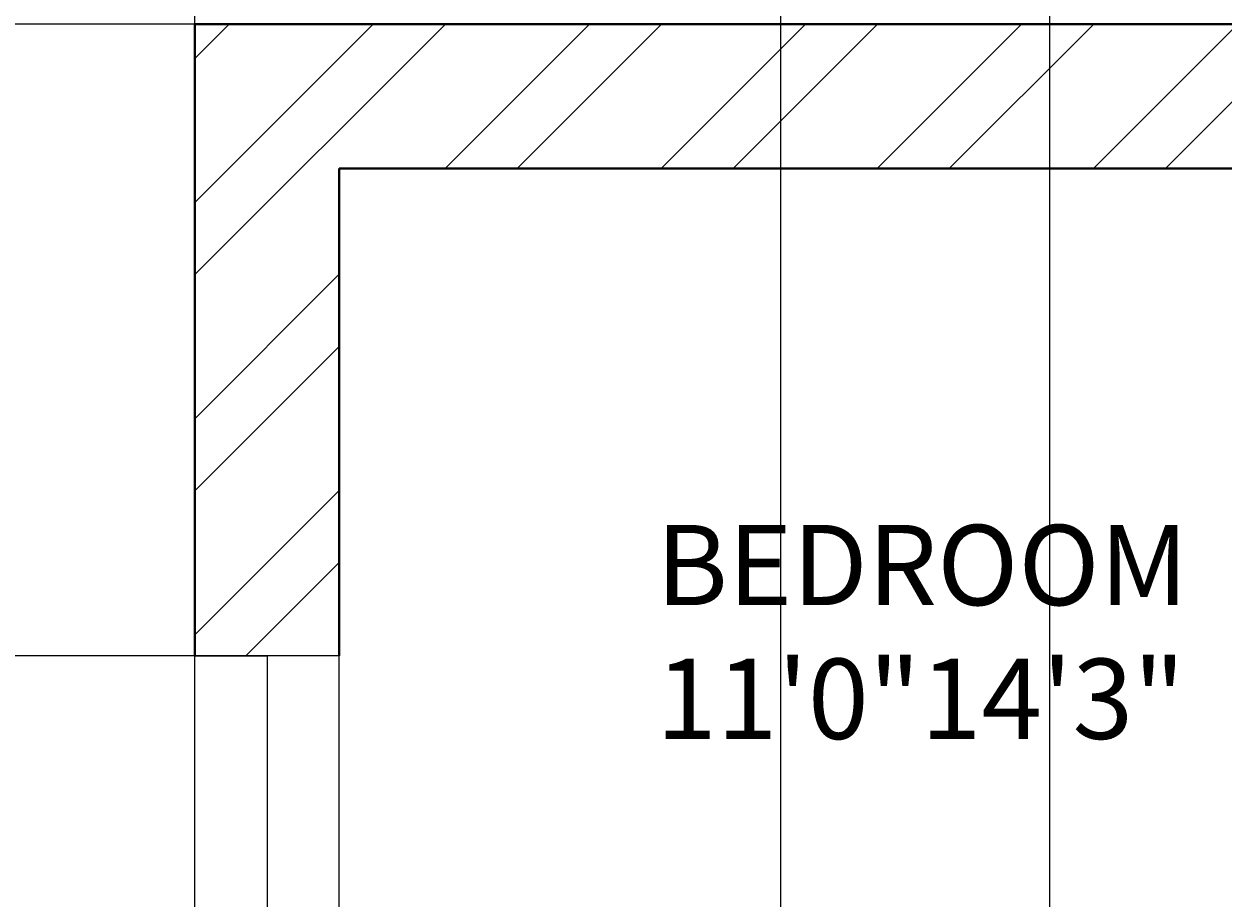
# Model space of a CAD drawing. Units: inches. Extents: x 1601 to 2297, y 1496 to 2631.
# Tile 40 of 57: x 1675 to 1750, y 2478 to 2532. Entities that reach past the tile are written whole.
import ezdxf

# ---------------------------------------------------------------- set-up
doc = ezdxf.new("R2010")
doc.units = ezdxf.units.IN
for name, color, linetype, lineweight in [('A-ANNO-DIMS', 2, 'Continuous', 18), ('A-AREA-IDEN', 7, 'Continuous', 18), ('A-GLAZ', 161, 'Continuous', 20), ('A-WALL', 7, 'Continuous', 40), ('A-WALL-PATT', 215, 'Continuous', 13)]:
    doc.layers.add(name, color=color, linetype=linetype, lineweight=lineweight)
doc.styles.get("Standard").update_dxf_attribs({"font": 'arial.ttf'})
doc.dimstyles.get("Standard").update_dxf_attribs({"dimtxt": 0.18, "dimasz": 0.18, "dimexe": 0.18, "dimexo": 0.0625, "dimgap": 0.09, "dimtad": 0, "dimtih": 1, "dimtoh": 1, "dimdec": 4, "dimzin": 0, "dimdsep": 46, "dimtxsty": 'Standard', "dimcen": 0.09, "dimadec": 0, "dimazin": 0, "dimtfac": 1, "dimtdec": 4, "dimtofl": 0, "dimtmove": 0, "dimatfit": 3, "dimfxl": 1, "dimtolj": 1, "dimtzin": 0, "dimarcsym": 0})

# ---------------------------------------------------------------- blocks, each defined once
blk = doc.blocks.new('WIN-60IN-JAMB9')
for p, q in [((4.5, 60), (0, 60)), ((0, 60), (9, 60)), ((0, 60), (0, 0)), ((4.5, 0), (4.5, 60)), ((9, 60), (9, 0)), ((0, 0), (9, 0)), ((9, 0), (4.5, 0))]:
    blk.add_line(p, q)
blk = doc.blocks.new('*D32')
at = {"layer": 'A-ANNO-DIMS', "color": 0, "lineweight": -2, "transparency": 16777216}
for p, q in [((1686.037, 2031.388), (1686.037, 2581.055)), ((1686.217, 2580.875), (1703.909, 2580.875)), ((1722.389, 2580.875), (1704.697, 2580.875)), ((1722.569, 2031.388), (1722.569, 2581.055))]:
    blk.add_line(p, q, dxfattribs=at)
at = {"layer": 'A-ANNO-DIMS', "color": 0, "transparency": 16777216}
for points in [[(1686.217, 2580.905), (1686.217, 2580.845), (1686.037, 2580.875)], [(1722.389, 2580.905), (1722.389, 2580.845), (1722.569, 2580.875)]]:
    blk.add_solid(points, dxfattribs=at)
at = {"layer": 'Defpoints', "color": 0, "transparency": 16777216}
for p in [(1722.569, 2580.875), (1686.037, 2031.325), (1722.569, 2031.325)]:
    blk.add_point(p, dxfattribs=at)
at = {"layer": 'A-ANNO-DIMS', "color": 0, "transparency": 16777216, "insert": (1704.303, 2580.875), "char_height": 0.18, "attachment_point": 5}
blk.add_mtext('\\A1;36.53', dxfattribs=at)
blk = doc.blocks.new('*D35')
at = {"layer": 'A-ANNO-DIMS', "color": 0, "lineweight": -2, "transparency": 16777216}
for p, q in [((1685.975, 2532.325), (1637.307, 2532.325)), ((1637.487, 2532.145), (1637.487, 2512.819)), ((1637.487, 2493.129), (1637.487, 2512.455)), ((1685.975, 2492.949), (1637.307, 2492.949))]:
    blk.add_line(p, q, dxfattribs=at)
at = {"layer": 'A-ANNO-DIMS', "color": 0, "transparency": 16777216}
for points in [[(1637.457, 2532.145), (1637.517, 2532.145), (1637.487, 2532.325)], [(1637.457, 2493.129), (1637.517, 2493.129), (1637.487, 2492.949)]]:
    blk.add_solid(points, dxfattribs=at)
at = {"layer": 'Defpoints', "color": 0, "transparency": 16777216}
for p in [(1637.487, 2532.325), (1686.037, 2532.325), (1686.037, 2492.949)]:
    blk.add_point(p, dxfattribs=at)
at = {"layer": 'A-ANNO-DIMS', "color": 0, "transparency": 16777216, "insert": (1637.487, 2512.637), "char_height": 0.18, "attachment_point": 5}
blk.add_mtext('\\A1;39.376', dxfattribs=at)
blk = doc.blocks.new('*D36')
at = {"layer": 'A-ANNO-DIMS', "color": 0, "lineweight": -2, "transparency": 16777216}
for p, q in [((1686.037, 1635.388), (1686.037, 2581.055)), ((1686.217, 2580.875), (1712.362, 2580.875)), ((1739.154, 2580.875), (1713.009, 2580.875)), ((1739.334, 1635.388), (1739.334, 2581.055))]:
    blk.add_line(p, q, dxfattribs=at)
at = {"layer": 'A-ANNO-DIMS', "color": 0, "transparency": 16777216}
for points in [[(1686.217, 2580.905), (1686.217, 2580.845), (1686.037, 2580.875)], [(1739.154, 2580.905), (1739.154, 2580.845), (1739.334, 2580.875)]]:
    blk.add_solid(points, dxfattribs=at)
at = {"layer": 'Defpoints', "color": 0, "transparency": 16777216}
for p in [(1739.334, 2580.875), (1686.037, 1635.325), (1739.334, 1635.325)]:
    blk.add_point(p, dxfattribs=at)
at = {"layer": 'A-ANNO-DIMS', "color": 0, "transparency": 16777216, "insert": (1712.685, 2580.875), "char_height": 0.18, "attachment_point": 5}
blk.add_mtext('\\A1;53.3', dxfattribs=at)

msp = doc.modelspace()

# ---------------------------------------------------------------- hatches: boundary and pattern name
at = {"layer": 'A-WALL-PATT'}
h = msp.add_hatch(dxfattribs=at)
h.set_pattern_fill('ANSI32', color=256)
h.paths.add_polyline_path([(1842.0336, 2528.0767), (1842.0336, 2532.3254), (1686.0373, 2532.3254), (1686.0373, 2492.9493), (1695.0373, 2492.9493), (1695.0373, 2523.3254), (1827.0373, 2523.3254), (1827.0373, 2416.8254), (1834.6225, 2416.8254), (1834.6225, 2419.0754), (1834.6225, 2421.3254), (1831.5373, 2421.3254), (1831.5373, 2523.3254), (1842.0336, 2523.3254)])
h.paths.add_polyline_path([(1695.0373, 2432.9493), (1686.0373, 2432.9493), (1686.0373, 2325.989), (1695.0373, 2325.989), (1695.0373, 2347.8254), (1827.0373, 2347.8254), (1827.0373, 2287.8254), (1823.2991, 2287.8254), (1823.2991, 2283.3254), (1847.9422, 2283.3254), (1847.9422, 2285.5754), (1847.9422, 2287.8254), (1831.5373, 2287.8254), (1831.5373, 2347.8254), (1846.9946, 2347.8254), (1846.9946, 2350.0754), (1846.9946, 2352.3254), (1695.0373, 2352.3254)])
h.paths.add_polyline_path([(1807.1169, 1573.5395), (2055.0405, 1573.5395), (2055.0405, 1610.6322), (1807.1169, 1610.6322)], flags=9)
h.paths.add_polyline_path([(1841.1631, 1712.7967), (1870.3957, 1712.7967), (1870.3957, 1731.454), (1841.1631, 1731.454)], flags=9)
h.paths.add_polyline_path([(2144.3862, 1772.185), (2191.0233, 1772.185), (2191.0233, 1790.8423), (2144.3862, 1790.8423)], flags=9)
h.paths.add_polyline_path([(2143.0128, 1827.3312), (2177.9958, 1827.3312), (2177.9958, 1845.9886), (2143.0128, 1845.9886)], flags=9)
h.paths.add_polyline_path([(2041.2439, 1833.5691), (2070.8516, 1833.5691), (2070.8516, 1852.2264), (2041.2439, 1852.2264)], flags=9)
h.paths.add_polyline_path([(2097.2791, 1947.0598), (2134.2061, 1947.0598), (2134.2061, 1965.7171), (2097.2791, 1965.7171)], flags=9)
h.paths.add_polyline_path([(2214.995, 1904.3124), (2214.995, 1942.2899), (2196.3376, 1942.2899), (2196.3376, 1904.3124)], flags=9)
h.paths.add_polyline_path([(2186.6284, 2043.8031), (2219.7935, 2043.8031), (2219.7935, 2062.4605), (2186.6284, 2062.4605)], flags=9)
h.paths.add_polyline_path([(2064.0877, 2031.616), (2097.4949, 2031.616), (2097.4949, 2050.2734), (2064.0877, 2050.2734)], flags=9)
h.paths.add_polyline_path([(1973.1349, 1986.0688), (2008.4009, 1986.0688), (2008.4009, 2004.7261), (1973.1349, 2004.7261)], flags=9)
h.paths.add_polyline_path([(1976.3676, 2106.9635), (2005.7469, 2106.9635), (2005.7469, 2125.6209), (1976.3676, 2125.6209)], flags=9)
h.paths.add_polyline_path([(1991.7852, 2180.4863), (2027.0513, 2180.4863), (2027.0513, 2199.1437), (1991.7852, 2199.1437)], flags=9)
h.paths.add_polyline_path([(2106.1801, 2187.9359), (2152.2101, 2187.9359), (2152.2101, 2206.5932), (2106.1801, 2206.5932)], flags=9)
h.paths.add_polyline_path([(2148.6686, 2262.2542), (2182.318, 2262.2542), (2182.318, 2280.9115), (2148.6686, 2280.9115)], flags=9)
h.paths.add_polyline_path([(2041.6327, 2252.8147), (2071.2405, 2252.8147), (2071.2405, 2271.4721), (2041.6327, 2271.4721)], flags=9)
h.paths.add_polyline_path([(2063.9734, 2375.4265), (2100.9004, 2375.4265), (2100.9004, 2394.0839), (2063.9734, 2394.0839)], flags=9)
h.paths.add_polyline_path([(2216.4955, 2330.9748), (2216.4955, 2370.2654), (2197.8381, 2370.2654), (2197.8381, 2330.9748)], flags=9)
h.paths.add_polyline_path([(2179.1416, 2485.8687), (2212.3067, 2485.8687), (2212.3067, 2504.5261), (2179.1416, 2504.5261)], flags=9)
h.paths.add_polyline_path([(2078.7442, 2471.1516), (2112.1514, 2471.1516), (2112.1514, 2489.809), (2078.7442, 2489.809)], flags=9)
h.paths.add_polyline_path([(1915.9631, 2329.4668), (1952.8902, 2329.4668), (1952.8902, 2348.1241), (1915.9631, 2348.1241)], flags=9)
h.paths.add_polyline_path([(1904.3189, 2499.6709), (1940.4512, 2499.6709), (1940.4512, 2518.3282), (1904.3189, 2518.3282)], flags=9)
h.paths.add_polyline_path([(1892.3665, 2100.4595), (1925.6374, 2100.4595), (1925.6374, 2119.1169), (1892.3665, 2119.1169)], flags=9)
h.paths.add_polyline_path([(1909.2984, 1805.9631), (1946.2254, 1805.9631), (1946.2254, 1824.6205), (1909.2984, 1824.6205)], flags=9)
h.paths.add_polyline_path([(1934.6056, 1658.616), (1970.738, 1658.616), (1970.738, 1677.2733), (1934.6056, 1677.2733)], flags=9)
h.paths.add_polyline_path([(1711.2052, 1789.8902), (1750.0456, 1789.8902), (1750.0456, 1808.5476), (1711.2052, 1808.5476)], flags=9)
h.paths.add_polyline_path([(1742.7874, 1854.6743), (1771.9449, 1854.6743), (1771.9449, 1873.3317), (1742.7874, 1873.3317)], flags=9)
h.paths.add_polyline_path([(1807.3592, 1997.7912), (1850.1116, 1997.7912), (1850.1116, 2016.4486), (1807.3592, 2016.4486)], flags=9)
h.paths.add_polyline_path([(1717.4579, 2237.7844), (1760.2103, 2237.7844), (1760.2103, 2256.4417), (1717.4579, 2256.4417)], flags=9)
h.paths.add_polyline_path([(1780.9285, 2324.0623), (1810.086, 2324.0623), (1810.086, 2342.7197), (1780.9285, 2342.7197)], flags=25)
h.paths.add_polyline_path([(1837.696, 2449.2024), (1866.9286, 2449.2024), (1866.9286, 2467.8598), (1837.696, 2467.8598)], flags=9)
h.paths.add_polyline_path([(1712.7752, 2484.9404), (1751.6156, 2484.9404), (1751.6156, 2503.5977), (1712.7752, 2503.5977)], flags=25)
h = msp.add_hatch(dxfattribs=at)
h.set_pattern_fill('ANSI32', color=256)
h.paths.add_polyline_path([(1973.9371, 2211.3254), (1893.0373, 2211.3254), (1893.0373, 2287.8254), (1884.6167, 2287.8254), (1884.6167, 2285.5754), (1884.6167, 2283.3254), (1888.5373, 2283.3254), (1888.5373, 2145.3254), (1695.0373, 2145.3254), (1695.0373, 2173.8724), (1690.5373, 2173.8724), (1686.0373, 2173.8724), (1686.0373, 2136.3254), (1722.5687, 2136.3254), (1722.5687, 2117.4352), (1731.5687, 2117.4352), (1731.5687, 2136.3254), (1893.0373, 2136.3254), (1893.0373, 2202.3254), (1959.0373, 2202.3254), (1959.0373, 2182.1303), (1968.0373, 2182.1303), (1968.0373, 2202.3254), (1973.9371, 2202.3254)])
h.paths.add_polyline_path([(2094.0373, 2274.6364), (2096.4294, 2274.6364), (2096.4294, 2276.8864), (2096.4294, 2279.1364), (2094.0373, 2279.1364), (2094.0373, 2290.8254), (2094.0373, 2295.3254), (2089.5373, 2295.3254), (2089.5373, 2230.8254), (2035.5373, 2230.8254), (2035.5373, 2299.8254), (2031.0373, 2299.8254), (2031.0373, 2211.3254), (2023.0065, 2211.3254), (2023.0065, 2202.3254), (2031.0373, 2202.3254), (2031.0373, 2140.8254), (1968.0373, 2140.8254), (1968.0373, 2145.9106), (1963.5373, 2145.9106), (1959.0373, 2145.9106), (1959.0373, 2116.839), (1963.5373, 2116.839), (1968.0373, 2116.839), (1968.0373, 2131.8254), (2031.0373, 2131.8254), (2031.0373, 2094.3254), (2031.0373, 2085.3254), (2031.0373, 2056.8254), (1968.0373, 2056.8254), (1968.0373, 2070.4947), (1963.5373, 2070.4947), (1959.0373, 2070.4947), (1959.0373, 2040.3029), (1968.0373, 2040.3029), (1968.0373, 2047.8254), (2031.0373, 2047.8254), (2031.0373, 1983.3254), (2031.0373, 1978.8254), (2021.1979, 1978.8254), (2021.1979, 1974.3254), (2031.0373, 1974.3254), (2031.0373, 1954.3528), (2035.5373, 1954.3528), (2035.5373, 1974.3254), (2035.5373, 1981.8254), (2055.5513, 1981.8254), (2055.5513, 1986.3254), (2035.5373, 1986.3254), (2035.5373, 2047.8254), (2040.0373, 2047.8254), (2040.0373, 2085.3254), (2040.0373, 2094.3254), (2040.0373, 2140.8254), (2035.5373, 2140.8254), (2035.5373, 2226.3254), (2089.5373, 2226.3254), (2094.0373, 2226.3254)])
h.paths.add_polyline_path([(2226.0373, 2230.8254), (2134.5373, 2230.8254), (2134.5373, 2233.5437), (2130.0373, 2233.5437), (2130.0373, 2226.3254), (2134.5373, 2226.3254), (2226.0373, 2226.3254)])
h.paths.add_polyline_path([(1807.1169, 1573.5395), (2055.0405, 1573.5395), (2055.0405, 1610.6322), (1807.1169, 1610.6322)], flags=9)
h.paths.add_polyline_path([(1841.1631, 1712.7967), (1870.3957, 1712.7967), (1870.3957, 1731.454), (1841.1631, 1731.454)], flags=9)
h.paths.add_polyline_path([(2144.3862, 1772.185), (2191.0233, 1772.185), (2191.0233, 1790.8423), (2144.3862, 1790.8423)], flags=9)
h.paths.add_polyline_path([(2143.0128, 1827.3312), (2177.9958, 1827.3312), (2177.9958, 1845.9886), (2143.0128, 1845.9886)], flags=9)
h.paths.add_polyline_path([(2041.2439, 1833.5691), (2070.8516, 1833.5691), (2070.8516, 1852.2264), (2041.2439, 1852.2264)], flags=9)
h.paths.add_polyline_path([(2097.2791, 1947.0598), (2134.2061, 1947.0598), (2134.2061, 1965.7171), (2097.2791, 1965.7171)], flags=9)
h.paths.add_polyline_path([(2214.995, 1904.3124), (2214.995, 1942.2899), (2196.3376, 1942.2899), (2196.3376, 1904.3124)], flags=9)
h.paths.add_polyline_path([(2186.6284, 2043.8031), (2219.7935, 2043.8031), (2219.7935, 2062.4605), (2186.6284, 2062.4605)], flags=9)
h.paths.add_polyline_path([(2064.0877, 2031.616), (2097.4949, 2031.616), (2097.4949, 2050.2734), (2064.0877, 2050.2734)], flags=9)
h.paths.add_polyline_path([(1973.1349, 1986.0688), (2008.4009, 1986.0688), (2008.4009, 2004.7261), (1973.1349, 2004.7261)], flags=25)
h.paths.add_polyline_path([(1976.3676, 2106.9635), (2005.7469, 2106.9635), (2005.7469, 2125.6209), (1976.3676, 2125.6209)], flags=25)
h.paths.add_polyline_path([(1991.7852, 2180.4863), (2027.0513, 2180.4863), (2027.0513, 2199.1437), (1991.7852, 2199.1437)], flags=25)
h.paths.add_polyline_path([(2106.1801, 2187.9359), (2152.2101, 2187.9359), (2152.2101, 2206.5932), (2106.1801, 2206.5932)], flags=9)
h.paths.add_polyline_path([(2148.6686, 2262.2542), (2182.318, 2262.2542), (2182.318, 2280.9115), (2148.6686, 2280.9115)], flags=9)
h.paths.add_polyline_path([(2041.6327, 2252.8147), (2071.2405, 2252.8147), (2071.2405, 2271.4721), (2041.6327, 2271.4721)], flags=25)
h.paths.add_polyline_path([(2063.9734, 2375.4265), (2100.9004, 2375.4265), (2100.9004, 2394.0839), (2063.9734, 2394.0839)], flags=9)
h.paths.add_polyline_path([(2216.4955, 2330.9748), (2216.4955, 2370.2654), (2197.8381, 2370.2654), (2197.8381, 2330.9748)], flags=9)
h.paths.add_polyline_path([(2179.1416, 2485.8687), (2212.3067, 2485.8687), (2212.3067, 2504.5261), (2179.1416, 2504.5261)], flags=9)
h.paths.add_polyline_path([(2078.7442, 2471.1516), (2112.1514, 2471.1516), (2112.1514, 2489.809), (2078.7442, 2489.809)], flags=9)
h.paths.add_polyline_path([(1915.9631, 2329.4668), (1952.8902, 2329.4668), (1952.8902, 2348.1241), (1915.9631, 2348.1241)], flags=9)
h.paths.add_polyline_path([(1904.3189, 2499.6709), (1940.4512, 2499.6709), (1940.4512, 2518.3282), (1904.3189, 2518.3282)], flags=9)
h.paths.add_polyline_path([(1892.3665, 2100.4595), (1925.6374, 2100.4595), (1925.6374, 2119.1169), (1892.3665, 2119.1169)], flags=9)
h.paths.add_polyline_path([(1909.2984, 1805.9631), (1946.2254, 1805.9631), (1946.2254, 1824.6205), (1909.2984, 1824.6205)], flags=9)
h.paths.add_polyline_path([(1934.6056, 1658.616), (1970.738, 1658.616), (1970.738, 1677.2733), (1934.6056, 1677.2733)], flags=9)
h.paths.add_polyline_path([(1711.2052, 1789.8902), (1750.0456, 1789.8902), (1750.0456, 1808.5476), (1711.2052, 1808.5476)], flags=9)
h.paths.add_polyline_path([(1742.7874, 1854.6743), (1771.9449, 1854.6743), (1771.9449, 1873.3317), (1742.7874, 1873.3317)], flags=9)
h.paths.add_polyline_path([(1807.3592, 1997.7912), (1850.1116, 1997.7912), (1850.1116, 2016.4486), (1807.3592, 2016.4486)], flags=9)
h.paths.add_polyline_path([(1717.4579, 2237.7844), (1760.2103, 2237.7844), (1760.2103, 2256.4417), (1717.4579, 2256.4417)], flags=25)
h.paths.add_polyline_path([(1780.9285, 2324.0623), (1810.086, 2324.0623), (1810.086, 2342.7197), (1780.9285, 2342.7197)], flags=9)
h.paths.add_polyline_path([(1837.696, 2449.2024), (1866.9286, 2449.2024), (1866.9286, 2467.8598), (1837.696, 2467.8598)], flags=9)
h.paths.add_polyline_path([(1712.7752, 2484.9404), (1751.6156, 2484.9404), (1751.6156, 2503.5977), (1712.7752, 2503.5977)], flags=9)
h = msp.add_hatch(dxfattribs=at)
h.set_pattern_fill('ANSI32', color=256)
h.paths.add_polyline_path([(2230.5373, 1861.8254), (2182.5373, 1861.8254), (2182.5373, 1885.3637), (2178.0373, 1885.3637), (2178.0373, 1861.8254), (2166.0373, 1861.8254), (2134.5373, 1861.8254), (2130.0373, 1861.8254), (2130.0373, 1841.4682), (2126.8833, 1841.4682), (2126.8833, 1836.9682), (2130.0373, 1836.9682), (2130.0373, 1822.7302), (2134.5373, 1822.7302), (2134.5373, 1857.3254), (2166.0373, 1857.3254), (2226.0373, 1857.3254), (2226.0373, 1846.1155), (2230.5373, 1846.1155)])
h.paths.add_polyline_path([(2226.0373, 1797.3254), (2134.5373, 1797.3254), (2134.5373, 1800.6636), (2132.2873, 1800.6636), (2130.0373, 1800.6636), (2130.0373, 1797.3254), (2130.0373, 1792.8254), (2167.7264, 1792.8254), (2226.0373, 1792.8254)])
h.paths.add_polyline_path([(2230.5373, 1822.1155), (2226.0373, 1822.1155), (2226.0373, 1760.8563), (2230.5373, 1760.8563)])
h.paths.add_polyline_path([(2230.5373, 1700.8563), (2226.0373, 1700.8563), (2226.0373, 1644.3254), (2140.2517, 1644.3254), (2140.2517, 1635.3254), (2230.5373, 1635.3254)])
h.paths.add_polyline_path([(2080.2517, 1639.8254), (2080.2517, 1644.3254), (2035.5373, 1644.3254), (2035.5373, 1792.8254), (2094.0373, 1792.8254), (2094.0373, 1797.3254), (2094.0373, 1836.9682), (2097.1057, 1836.9682), (2097.1057, 1839.2182), (2097.1057, 1841.4682), (2094.0373, 1841.4682), (2094.0373, 1862.2276), (2089.5373, 1862.2276), (2089.5373, 1797.3254), (2035.5373, 1797.3254), (2035.5373, 1857.3254), (2035.5373, 1885.0916), (2031.0373, 1885.0916), (2031.0373, 1710.3254), (2012.329, 1710.3254), (2012.329, 1701.3254), (2031.0373, 1701.3254), (2031.0373, 1644.3254), (2031.0373, 1635.3254), (2080.2517, 1635.3254)])
h.paths.add_polyline_path([(1836.0373, 1653.2033), (1842.6171, 1653.2033), (1842.6171, 1657.7033), (1842.6171, 1662.2033), (1831.5373, 1662.2033), (1831.5373, 1764.2033), (1835.3881, 1764.2033), (1835.3881, 1766.4533), (1835.3881, 1768.7033), (1831.5373, 1768.7033), (1827.0373, 1768.7033), (1827.0373, 1662.2033), (1827.0373, 1635.3254), (1836.0373, 1635.3254)])
h.paths.add_polyline_path([(1893.0373, 1701.3254), (1907.193, 1701.3254), (1907.193, 1705.8254), (1907.193, 1710.3254), (1893.0373, 1710.3254), (1893.0373, 1819.8254), (1882.6444, 1819.8254), (1882.6444, 1817.5754), (1882.6444, 1815.3254), (1888.5373, 1815.3254), (1888.5373, 1662.2033), (1884.0373, 1662.2033), (1866.6171, 1662.2033), (1866.6171, 1653.2033), (1882.391, 1653.2033), (1884.0373, 1653.2033), (1884.0373, 1635.3254), (1893.0373, 1635.3254)])
h.paths.add_polyline_path([(1739.3335, 1639.8254), (1739.3335, 1644.3254), (1695.0373, 1644.3254), (1695.0373, 1702.0135), (1690.5373, 1702.0135), (1686.0373, 1702.0135), (1686.0373, 1635.3254), (1739.3335, 1635.3254)])
h.paths.add_polyline_path([(1827.0373, 1644.3254), (1799.3335, 1644.3254), (1799.3335, 1635.3254), (1827.0373, 1635.3254)])
h.paths.add_polyline_path([(1695.0373, 1815.3254), (1849.2759, 1815.3254), (1849.2759, 1819.8254), (1807.5373, 1819.8254), (1807.5373, 1879.8254), (1851.1533, 1879.8254), (1851.1533, 1882.0754), (1851.1533, 1884.3254), (1799.3405, 1884.3254), (1799.3405, 1882.0754), (1799.3405, 1879.8254), (1803.0373, 1879.8254), (1803.0373, 1819.8254), (1695.0373, 1819.8254), (1695.0373, 1835.0458), (1690.5373, 1835.0458), (1686.0373, 1835.0458), (1686.0373, 1766.1753), (1695.0373, 1766.1753)])
h.paths.add_polyline_path([(1775.8157, 1884.3254), (1695.0373, 1884.3254), (1695.0373, 1912.9526), (1690.5373, 1912.9526), (1686.0373, 1912.9526), (1686.0373, 1859.0458), (1695.0373, 1859.0458), (1695.0373, 1879.8254), (1775.8157, 1879.8254)])
h.paths.add_polyline_path([(1893.0373, 2031.3254), (1731.5687, 2031.3254), (1731.5687, 2057.4352), (1722.5687, 2057.4352), (1722.5687, 2031.3254), (1686.0373, 2031.3254), (1686.0373, 1972.9526), (1695.0373, 1972.9526), (1695.0373, 2022.3254), (1888.5373, 2022.3254), (1888.5373, 1884.3254), (1883.4996, 1884.3254), (1883.4996, 1879.8254), (1893.0373, 1879.8254), (1893.0373, 1974.3254), (1976.6199, 1974.3254), (1976.6199, 1978.8254), (1968.0373, 1978.8254), (1968.0373, 1983.3254), (1968.0373, 2008.4756), (1963.5373, 2008.4756), (1959.0373, 2008.4756), (1959.0373, 1983.3254), (1893.0373, 1983.3254)])
h.paths.add_polyline_path([(2230.5373, 2140.4745), (2226.0373, 2140.4745), (2226.0373, 2094.3254), (2040.0373, 2094.3254), (2040.0373, 2085.3254), (2178.0373, 2085.3254), (2178.0373, 2065.6965), (2182.5373, 2065.6965), (2182.5373, 2085.3254), (2226.0373, 2085.3254), (2226.0373, 1986.3254), (2211.2679, 1986.3254), (2211.2679, 1981.8254), (2230.5373, 1981.8254)])
h.paths.add_polyline_path([(2187.6292, 1986.3254), (2182.5373, 1986.3254), (2182.5373, 2029.6965), (2178.0373, 2029.6965), (2178.0373, 1986.3254), (2099.05, 1986.3254), (2099.05, 1981.8254), (2178.0373, 1981.8254), (2178.0373, 1969.3637), (2182.5373, 1969.3637), (2182.5373, 1981.8254), (2187.6292, 1981.8254), (2187.6292, 1984.0754)])
h.paths.add_polyline_path([(1807.1169, 1573.5395), (2055.0405, 1573.5395), (2055.0405, 1610.6322), (1807.1169, 1610.6322)], flags=9)
h.paths.add_polyline_path([(1841.1631, 1712.7967), (1870.3957, 1712.7967), (1870.3957, 1731.454), (1841.1631, 1731.454)], flags=9)
h.paths.add_polyline_path([(2144.3862, 1772.185), (2191.0233, 1772.185), (2191.0233, 1790.8423), (2144.3862, 1790.8423)], flags=9)
h.paths.add_polyline_path([(2143.0128, 1827.3312), (2177.9958, 1827.3312), (2177.9958, 1845.9886), (2143.0128, 1845.9886)], flags=25)
h.paths.add_polyline_path([(2041.2439, 1833.5691), (2070.8516, 1833.5691), (2070.8516, 1852.2264), (2041.2439, 1852.2264)], flags=25)
h.paths.add_polyline_path([(2097.2791, 1947.0598), (2134.2061, 1947.0598), (2134.2061, 1965.7171), (2097.2791, 1965.7171)], flags=9)
h.paths.add_polyline_path([(2214.995, 1904.3124), (2214.995, 1942.2899), (2196.3376, 1942.2899), (2196.3376, 1904.3124)], flags=9)
h.paths.add_polyline_path([(2186.6284, 2043.8031), (2219.7935, 2043.8031), (2219.7935, 2062.4605), (2186.6284, 2062.4605)], flags=25)
h.paths.add_polyline_path([(2064.0877, 2031.616), (2097.4949, 2031.616), (2097.4949, 2050.2734), (2064.0877, 2050.2734)], flags=25)
h.paths.add_polyline_path([(1973.1349, 1986.0688), (2008.4009, 1986.0688), (2008.4009, 2004.7261), (1973.1349, 2004.7261)], flags=9)
h.paths.add_polyline_path([(1976.3676, 2106.9635), (2005.7469, 2106.9635), (2005.7469, 2125.6209), (1976.3676, 2125.6209)], flags=9)
h.paths.add_polyline_path([(1991.7852, 2180.4863), (2027.0513, 2180.4863), (2027.0513, 2199.1437), (1991.7852, 2199.1437)], flags=9)
h.paths.add_polyline_path([(2106.1801, 2187.9359), (2152.2101, 2187.9359), (2152.2101, 2206.5932), (2106.1801, 2206.5932)], flags=9)
h.paths.add_polyline_path([(2148.6686, 2262.2542), (2182.318, 2262.2542), (2182.318, 2280.9115), (2148.6686, 2280.9115)], flags=9)
h.paths.add_polyline_path([(2041.6327, 2252.8147), (2071.2405, 2252.8147), (2071.2405, 2271.4721), (2041.6327, 2271.4721)], flags=9)
h.paths.add_polyline_path([(2063.9734, 2375.4265), (2100.9004, 2375.4265), (2100.9004, 2394.0839), (2063.9734, 2394.0839)], flags=9)
h.paths.add_polyline_path([(2216.4955, 2330.9748), (2216.4955, 2370.2654), (2197.8381, 2370.2654), (2197.8381, 2330.9748)], flags=9)
h.paths.add_polyline_path([(2179.1416, 2485.8687), (2212.3067, 2485.8687), (2212.3067, 2504.5261), (2179.1416, 2504.5261)], flags=9)
h.paths.add_polyline_path([(2078.7442, 2471.1516), (2112.1514, 2471.1516), (2112.1514, 2489.809), (2078.7442, 2489.809)], flags=9)
h.paths.add_polyline_path([(1915.9631, 2329.4668), (1952.8902, 2329.4668), (1952.8902, 2348.1241), (1915.9631, 2348.1241)], flags=9)
h.paths.add_polyline_path([(1904.3189, 2499.6709), (1940.4512, 2499.6709), (1940.4512, 2518.3282), (1904.3189, 2518.3282)], flags=9)
h.paths.add_polyline_path([(1892.3665, 2100.4595), (1925.6374, 2100.4595), (1925.6374, 2119.1169), (1892.3665, 2119.1169)], flags=9)
h.paths.add_polyline_path([(1909.2984, 1805.9631), (1946.2254, 1805.9631), (1946.2254, 1824.6205), (1909.2984, 1824.6205)], flags=9)
h.paths.add_polyline_path([(1934.6056, 1658.616), (1970.738, 1658.616), (1970.738, 1677.2733), (1934.6056, 1677.2733)], flags=9)
h.paths.add_polyline_path([(1711.2052, 1789.8902), (1750.0456, 1789.8902), (1750.0456, 1808.5476), (1711.2052, 1808.5476)], flags=25)
h.paths.add_polyline_path([(1742.7874, 1854.6743), (1771.9449, 1854.6743), (1771.9449, 1873.3317), (1742.7874, 1873.3317)], flags=25)
h.paths.add_polyline_path([(1807.3592, 1997.7912), (1850.1116, 1997.7912), (1850.1116, 2016.4486), (1807.3592, 2016.4486)], flags=25)
h.paths.add_polyline_path([(1717.4579, 2237.7844), (1760.2103, 2237.7844), (1760.2103, 2256.4417), (1717.4579, 2256.4417)], flags=9)
h.paths.add_polyline_path([(1780.9285, 2324.0623), (1810.086, 2324.0623), (1810.086, 2342.7197), (1780.9285, 2342.7197)], flags=9)
h.paths.add_polyline_path([(1837.696, 2449.2024), (1866.9286, 2449.2024), (1866.9286, 2467.8598), (1837.696, 2467.8598)], flags=9)
h.paths.add_polyline_path([(1712.7752, 2484.9404), (1751.6156, 2484.9404), (1751.6156, 2503.5977), (1712.7752, 2503.5977)], flags=9)

# ---------------------------------------------------------------- linework, layer by layer
at = {"layer": 'A-WALL'}
for p, q in [((1686.0373, 2532.3254), (1842.0336, 2532.3254)), ((1686.0373, 2532.3254), (1686.0373, 2492.9493)), ((1695.0373, 2523.3254), (1827.0373, 2523.3254)), ((1695.0373, 2523.3254), (1695.0373, 2492.9493))]:
    msp.add_line(p, q, dxfattribs=at)

# ---------------------------------------------------------------- block references
at = {"layer": 'A-GLAZ', "rotation": 180}
msp.add_blockref('WIN-60IN-JAMB9', (1695.0376, 2492.9498), dxfattribs=at)

# ---------------------------------------------------------------- texts
at = {"layer": 'A-AREA-IDEN', "insert": (1714.7858, 2501.1131), "char_height": 5, "attachment_point": 1}
msp.add_mtext_dynamic_manual_height_columns('BEDROOM\\P11\'0"14\'3"', width=102.368064, gutter_width=12.5, heights=[0], dxfattribs=at)

# ---------------------------------------------------------------- dimensions: what is measured, and where the dimension line sits
at = {"layer": 'A-ANNO-DIMS'}
for base, p1, p2, override, picture, middle in [((1722.5687, 2580.8754), (1686.0373, 2031.3254), (1722.5687, 2031.3254), {"dimdec": 2, "dimlfac": 1, "dimrnd": 0, "dimzin": 0, "dimdsep": 46, "dimlunit": 2}, '*D32', (1704.303, 2580.8754)), ((1739.3335, 2580.8754), (1686.0373, 1635.3254), (1739.3335, 1635.3254), {"dimdec": 1, "dimlfac": 1, "dimrnd": 0, "dimzin": 0, "dimdsep": 46, "dimlunit": 2}, '*D36', (1712.6854, 2580.8754))]:
    dim = msp.add_linear_dim(base=base, p1=p1, p2=p2, dimstyle='Standard', override=override, dxfattribs=at)
    dim.commit()
    dim.dimension.update_dxf_attribs({"geometry": picture, "text_midpoint": middle})
dim = msp.add_linear_dim(base=(1637.4873, 2532.3254), p1=(1686.0373, 2492.9493), p2=(1686.0373, 2532.3254), angle=90, dimstyle='Standard', override={"dimdec": 3, "dimlfac": 1, "dimrnd": 0, "dimzin": 0, "dimdsep": 46, "dimlunit": 2}, dxfattribs=at)
dim.commit()
dim.dimension.update_dxf_attribs({"geometry": '*D35', "text_midpoint": (1637.4873, 2512.6374)})

doc.saveas('drawing.dxf')
